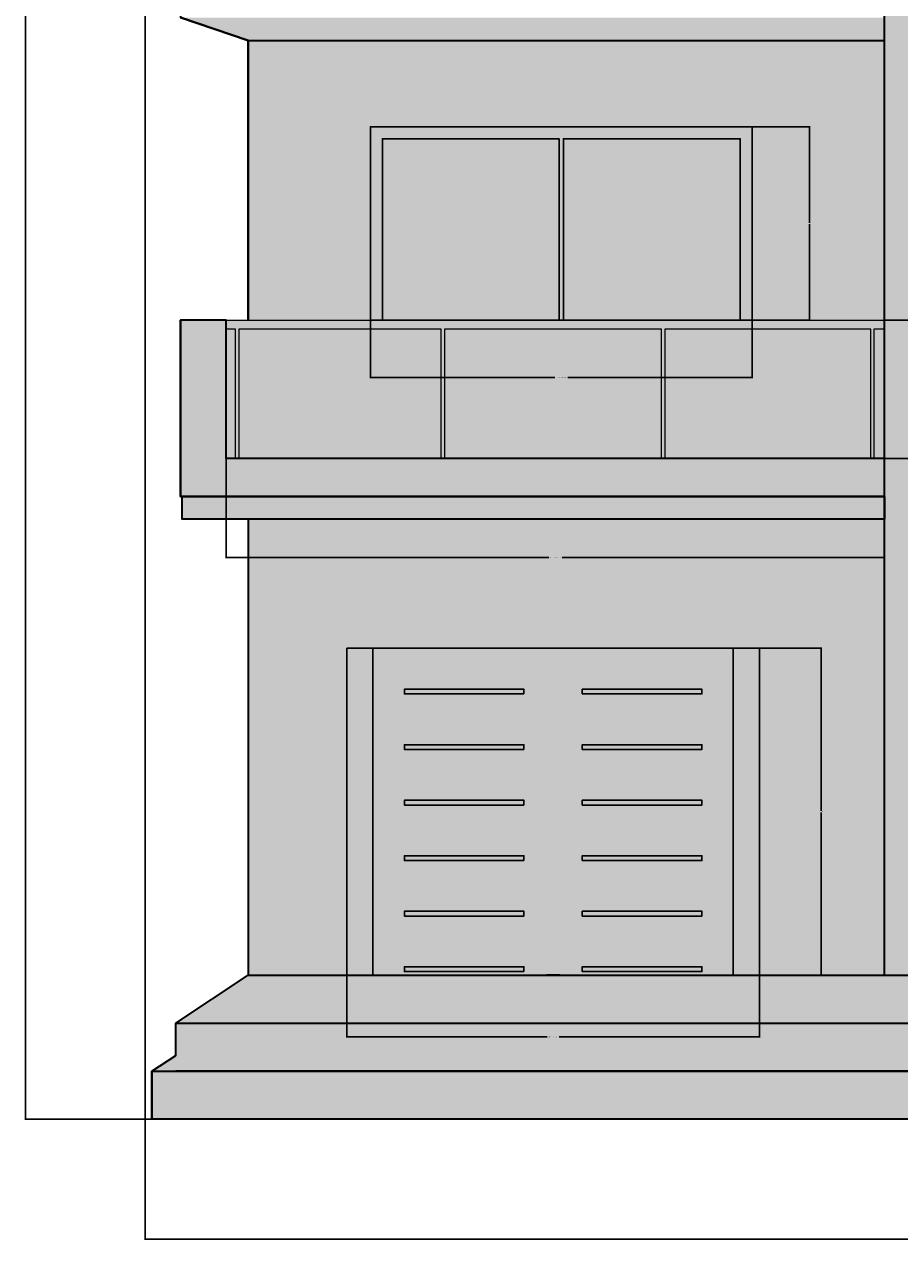
# Model space of a CAD drawing. Units: feet. Extents: x 2893 to 4112, y 897 to 1573.
# Tile 1 of 7: x 2893 to 3123, y 897 to 1217. Entities that reach past the tile are written whole.
import ezdxf

# ---------------------------------------------------------------- set-up
doc = ezdxf.new("R2010")
doc.units = ezdxf.units.FT
for name, color, linetype, lineweight in [('A-ANNO-DIMS', 2, 'Continuous', 18), ('A-DOOR', 3, 'Continuous', 25), ('A-ELEV', 7, 'Continuous', 35), ('A-ELEV-PATT', 8, 'Continuous', 13), ('A-ELEV-RAIL', 4, 'Continuous', 18), ('A-GLAZ', 4, 'Continuous', 25)]:
    doc.layers.add(name, color=color, linetype=linetype, lineweight=lineweight)
doc.styles.get("Standard").update_dxf_attribs({"font": 'arial.ttf'})
doc.dimstyles.get("Standard").update_dxf_attribs({"dimtxt": 0.18, "dimasz": 0.18, "dimexe": 0.18, "dimexo": 0.0625, "dimgap": 0.09, "dimtad": 0, "dimtih": 1, "dimtoh": 1, "dimdec": 1, "dimzin": 0, "dimdsep": 46, "dimlunit": 3, "dimtxsty": 'Standard', "dimcen": 0.09, "dimadec": 0, "dimazin": 0, "dimtfac": 1, "dimtdec": 1, "dimtofl": 0, "dimtmove": 0, "dimatfit": 3, "dimfxl": 1, "dimtolj": 1, "dimtzin": 0, "dimarcsym": 0})

# ---------------------------------------------------------------- blocks, each defined once
blk = doc.blocks.new('WIN-SLIDING')
blk.add_lwpolyline([(100.48, 0), (0, 0), (0, 50.91), (100.48, 50.91)], close=True)
blk.add_lwpolyline([(100.48, 0), (0, 0), (0, 50.91), (100.48, 50.91)], close=True)
blk.add_lwpolyline([(97.33, 0), (97.33, 47.76), (50.81, 47.76), (50.81, 0), (49.67, 0), (49.67, 47.76), (3.15, 47.76), (3.15, 0)])
blk.add_lwpolyline([(97.33, 0), (97.33, 47.76), (50.81, 47.76), (50.81, 0), (49.67, 0), (49.67, 47.76), (3.15, 47.76), (3.15, 0)])
blk = doc.blocks.new('GATE-GARAGE')
for points in [[(108.58, 0), (0, 0), (0, 86.02), (108.58, 86.02)], [(108.58, 0), (0, 0), (0, 86.02), (108.58, 86.02)], [(0, 86.02), (6.87, 86.02), (6.87, 0), (0, 0)], [(0, 86.02), (6.87, 86.02), (6.87, 0), (0, 0)], [(108.58, 86.02), (101.71, 86.02), (101.71, 0), (108.58, 0)], [(108.58, 86.02), (101.71, 86.02), (101.71, 0), (108.58, 0)], [(46.6, 73.98), (15.13, 73.98), (15.13, 75.22), (46.6, 75.22)], [(46.6, 73.98), (15.13, 73.98), (15.13, 75.22), (46.6, 75.22)], [(61.97, 73.98), (93.45, 73.98), (93.45, 75.22), (61.97, 75.22)], [(61.97, 73.98), (93.45, 73.98), (93.45, 75.22), (61.97, 75.22)], [(46.6, 59.37), (15.13, 59.37), (15.13, 60.61), (46.6, 60.61)], [(46.6, 59.37), (15.13, 59.37), (15.13, 60.61), (46.6, 60.61)], [(61.97, 59.37), (93.45, 59.37), (93.45, 60.61), (61.97, 60.61)], [(61.97, 59.37), (93.45, 59.37), (93.45, 60.61), (61.97, 60.61)], [(46.6, 44.76), (15.13, 44.76), (15.13, 46), (46.6, 46)], [(46.6, 44.76), (15.13, 44.76), (15.13, 46), (46.6, 46)], [(61.97, 44.76), (93.45, 44.76), (93.45, 46), (61.97, 46)], [(61.97, 44.76), (93.45, 44.76), (93.45, 46), (61.97, 46)], [(46.6, 30.15), (15.13, 30.15), (15.13, 31.39), (46.6, 31.39)], [(46.6, 30.15), (15.13, 30.15), (15.13, 31.39), (46.6, 31.39)], [(61.97, 30.15), (93.45, 30.15), (93.45, 31.39), (61.97, 31.39)], [(61.97, 30.15), (93.45, 30.15), (93.45, 31.39), (61.97, 31.39)], [(46.6, 15.54), (15.13, 15.54), (15.13, 16.78), (46.6, 16.78)], [(46.6, 15.54), (15.13, 15.54), (15.13, 16.78), (46.6, 16.78)], [(61.97, 15.54), (93.45, 15.54), (93.45, 16.78), (61.97, 16.78)], [(61.97, 15.54), (93.45, 15.54), (93.45, 16.78), (61.97, 16.78)], [(46.6, 0.93), (15.13, 0.93), (15.13, 2.17), (46.6, 2.17)], [(46.6, 0.93), (15.13, 0.93), (15.13, 2.17), (46.6, 2.17)], [(61.97, 0.93), (93.45, 0.93), (93.45, 2.17), (61.97, 2.17)], [(61.97, 0.93), (93.45, 0.93), (93.45, 2.17), (61.97, 2.17)]]:
    blk.add_lwpolyline(points, close=True)
blk = doc.blocks.new('BALCONY-RAIL')
blk.add_lwpolyline([(56.56, 34.07), (3.3, 34.07), (3.3, 0), (2.43, 0), (2.43, 34.07), (0, 34.07), (0, 36.45), (173.25, 36.45), (173.25, 34.07), (170.48, 34.07), (170.48, 0), (169.61, 0), (169.61, 34.07), (115.47, 34.07), (115.47, 0), (114.59, 0), (114.59, 34.07), (57.43, 34.07), (57.43, 0), (56.56, 0)], close=True)
blk.add_lwpolyline([(56.56, 34.07), (3.3, 34.07), (3.3, 0), (2.43, 0), (2.43, 34.07), (0, 34.07), (0, 36.45), (173.25, 36.45), (173.25, 34.07), (170.48, 34.07), (170.48, 0), (169.61, 0), (169.61, 34.07), (115.47, 34.07), (115.47, 0), (114.59, 0), (114.59, 34.07), (57.43, 34.07), (57.43, 0), (56.56, 0)], close=True)
blk = doc.blocks.new('*D5')
at = {"layer": 'A-ANNO-DIMS', "color": 0, "lineweight": -2, "transparency": 16777216}
for p, q in [((2984.02, 1139.32), (2984.02, 1124.13)), ((3084.5, 1139.32), (3084.5, 1124.13)), ((2984.2, 1124.31), (3032.54, 1124.31)), ((3084.32, 1124.31), (3035.98, 1124.31))]:
    blk.add_line(p, q, dxfattribs=at)
at = {"layer": 'A-ANNO-DIMS', "color": 0, "transparency": 16777216}
for points in [[(2984.2, 1124.34), (2984.2, 1124.28), (2984.02, 1124.31)], [(3084.32, 1124.34), (3084.32, 1124.28), (3084.5, 1124.31)]]:
    blk.add_solid(points, dxfattribs=at)
at = {"layer": 'Defpoints', "color": 0, "transparency": 16777216}
for p in [(2984.02, 1139.38), (3084.5, 1139.38), (3084.5, 1124.31)]:
    blk.add_point(p, dxfattribs=at)
at = {"layer": 'A-ANNO-DIMS', "color": 0, "transparency": 16777216, "insert": (3034.26, 1124.31), "char_height": 0.18, "attachment_point": 5}
blk.add_mtext('\\A1;SLIDING WINDOW 100 TYP.', dxfattribs=at)
blk = doc.blocks.new('*D6')
at = {"layer": 'A-ANNO-DIMS', "color": 0, "lineweight": -2, "transparency": 16777216}
for p, q in [((3084.56, 1190.29), (3099.75, 1190.29)), ((3099.57, 1190.11), (3099.57, 1165.02)), ((3099.57, 1139.56), (3099.57, 1164.65)), ((3084.56, 1139.38), (3099.75, 1139.38))]:
    blk.add_line(p, q, dxfattribs=at)
at = {"layer": 'A-ANNO-DIMS', "color": 0, "transparency": 16777216}
for points in [[(3099.54, 1190.11), (3099.6, 1190.11), (3099.57, 1190.29)], [(3099.54, 1139.56), (3099.6, 1139.56), (3099.57, 1139.38)]]:
    blk.add_solid(points, dxfattribs=at)
at = {"layer": 'Defpoints', "color": 0, "transparency": 16777216}
for p in [(3084.5, 1190.29), (3099.57, 1190.29), (3084.5, 1139.38)]:
    blk.add_point(p, dxfattribs=at)
at = {"layer": 'A-ANNO-DIMS', "color": 0, "transparency": 16777216, "insert": (3099.57, 1164.84), "char_height": 0.18, "attachment_point": 5}
blk.add_mtext('\\A1;51 TYP.', dxfattribs=at)
blk = doc.blocks.new('*D7')
at = {"layer": 'A-ANNO-DIMS', "color": 0, "lineweight": -2, "transparency": 16777216}
for p, q in [((2946.08, 1102.87), (2946.08, 1076.76)), ((3119.33, 1102.87), (3119.33, 1076.76)), ((2946.26, 1076.94), (3030.93, 1076.94)), ((3119.15, 1076.94), (3034.47, 1076.94))]:
    blk.add_line(p, q, dxfattribs=at)
at = {"layer": 'A-ANNO-DIMS', "color": 0, "transparency": 16777216}
for points in [[(2946.26, 1076.97), (2946.26, 1076.91), (2946.08, 1076.94)], [(3119.15, 1076.97), (3119.15, 1076.91), (3119.33, 1076.94)]]:
    blk.add_solid(points, dxfattribs=at)
at = {"layer": 'Defpoints', "color": 0, "transparency": 16777216}
for p in [(2946.08, 1102.93), (3119.33, 1102.93), (3119.33, 1076.94)]:
    blk.add_point(p, dxfattribs=at)
at = {"layer": 'A-ANNO-DIMS', "color": 0, "transparency": 16777216, "insert": (3032.7, 1076.94), "char_height": 0.18, "attachment_point": 5}
blk.add_mtext('\\A1;BALCONY RAILING 173 TYP.', dxfattribs=at)
blk = doc.blocks.new('*D8')
at = {"layer": 'A-ANNO-DIMS', "color": 0, "lineweight": -2, "transparency": 16777216}
for p, q in [((3119.39, 1139.38), (3145.49, 1139.38)), ((3145.31, 1139.2), (3145.31, 1121.34)), ((3145.31, 1103.11), (3145.31, 1120.97)), ((3119.39, 1102.93), (3145.49, 1102.93))]:
    blk.add_line(p, q, dxfattribs=at)
at = {"layer": 'A-ANNO-DIMS', "color": 0, "transparency": 16777216}
for points in [[(3145.28, 1139.2), (3145.34, 1139.2), (3145.31, 1139.38)], [(3145.28, 1103.11), (3145.34, 1103.11), (3145.31, 1102.93)]]:
    blk.add_solid(points, dxfattribs=at)
at = {"layer": 'Defpoints', "color": 0, "transparency": 16777216}
for p in [(3119.33, 1139.38), (3145.31, 1139.38), (3119.33, 1102.93)]:
    blk.add_point(p, dxfattribs=at)
at = {"layer": 'A-ANNO-DIMS', "color": 0, "transparency": 16777216, "insert": (3145.31, 1121.16), "char_height": 0.18, "attachment_point": 5}
blk.add_mtext('\\A1;36 TYP.', dxfattribs=at)
blk = doc.blocks.new('*D11')
at = {"layer": 'A-ANNO-DIMS', "color": 0, "lineweight": -2, "transparency": 16777216}
for p, q in [((2977.81, 966.95), (2977.81, 950.55)), ((3086.39, 966.95), (3086.39, 950.55)), ((2977.99, 950.73), (3030.55, 950.73)), ((3086.21, 950.73), (3033.65, 950.73))]:
    blk.add_line(p, q, dxfattribs=at)
at = {"layer": 'A-ANNO-DIMS', "color": 0, "transparency": 16777216}
for points in [[(2977.99, 950.76), (2977.99, 950.7), (2977.81, 950.73)], [(3086.21, 950.76), (3086.21, 950.7), (3086.39, 950.73)]]:
    blk.add_solid(points, dxfattribs=at)
at = {"layer": 'Defpoints', "color": 0, "transparency": 16777216}
for p in [(2977.81, 967.01), (3086.39, 967.01), (3086.39, 950.73)]:
    blk.add_point(p, dxfattribs=at)
at = {"layer": 'A-ANNO-DIMS', "color": 0, "transparency": 16777216, "insert": (3032.1, 950.73), "char_height": 0.18, "attachment_point": 5}
blk.add_mtext('\\A1;GARAGE GATE 109 TYP.', dxfattribs=at)
blk = doc.blocks.new('*D12')
at = {"layer": 'A-ANNO-DIMS', "color": 0, "lineweight": -2, "transparency": 16777216}
for p, q in [((3086.45, 1053.04), (3102.86, 1053.04)), ((3102.68, 1052.86), (3102.68, 1010.21)), ((3102.68, 967.19), (3102.68, 1009.84)), ((3086.45, 967.01), (3102.86, 967.01))]:
    blk.add_line(p, q, dxfattribs=at)
at = {"layer": 'A-ANNO-DIMS', "color": 0, "transparency": 16777216}
for points in [[(3102.65, 1052.86), (3102.71, 1052.86), (3102.68, 1053.04)], [(3102.65, 967.19), (3102.71, 967.19), (3102.68, 967.01)]]:
    blk.add_solid(points, dxfattribs=at)
at = {"layer": 'Defpoints', "color": 0, "transparency": 16777216}
for p in [(3086.39, 1053.04), (3102.68, 1053.04), (3086.39, 967.01)]:
    blk.add_point(p, dxfattribs=at)
at = {"layer": 'A-ANNO-DIMS', "color": 0, "transparency": 16777216, "insert": (3102.68, 1010.03), "char_height": 0.18, "attachment_point": 5}
blk.add_mtext('\\A1;86 TYP.', dxfattribs=at)
blk = doc.blocks.new('*D48')
at = {"layer": 'A-ANNO-DIMS', "color": 0, "lineweight": -2, "transparency": 16777216}
for p, q in [((2924.72, 1491.83), (2924.72, 897.37)), ((3417.56, 1491.83), (3417.56, 897.37)), ((2924.9, 897.55), (3170.74, 897.55)), ((3417.38, 897.55), (3171.54, 897.55))]:
    blk.add_line(p, q, dxfattribs=at)
at = {"layer": 'A-ANNO-DIMS', "color": 0, "transparency": 16777216}
for points in [[(2924.9, 897.58), (2924.9, 897.52), (2924.72, 897.55)], [(3417.38, 897.58), (3417.38, 897.52), (3417.56, 897.55)]]:
    blk.add_solid(points, dxfattribs=at)
at = {"layer": 'Defpoints', "color": 0, "transparency": 16777216}
for p in [(2924.72, 1491.89), (3417.56, 1491.89), (3417.56, 897.55)]:
    blk.add_point(p, dxfattribs=at)
at = {"layer": 'A-ANNO-DIMS', "color": 0, "transparency": 16777216, "insert": (3171.14, 897.55), "char_height": 0.18, "attachment_point": 5}
blk.add_mtext('\\A1;492.8', dxfattribs=at)
blk = doc.blocks.new('*D55')
at = {"layer": 'A-ANNO-DIMS', "color": 0, "lineweight": -2, "transparency": 16777216}
for p, q in [((2924.66, 1527.89), (2893.04, 1527.89)), ((2893.22, 1527.71), (2893.22, 1228.65)), ((2893.22, 929.23), (2893.22, 1228.29)), ((2926.44, 929.05), (2893.04, 929.05))]:
    blk.add_line(p, q, dxfattribs=at)
at = {"layer": 'A-ANNO-DIMS', "color": 0, "transparency": 16777216}
for points in [[(2893.19, 1527.71), (2893.25, 1527.71), (2893.22, 1527.89)], [(2893.19, 929.23), (2893.25, 929.23), (2893.22, 929.05)]]:
    blk.add_solid(points, dxfattribs=at)
at = {"layer": 'Defpoints', "color": 0, "transparency": 16777216}
for p in [(2893.22, 1527.89), (2924.72, 1527.89), (2926.51, 929.05)]:
    blk.add_point(p, dxfattribs=at)
at = {"layer": 'A-ANNO-DIMS', "color": 0, "transparency": 16777216, "insert": (2893.22, 1228.47), "char_height": 0.18, "attachment_point": 5}
blk.add_mtext('\\A1;598.8', dxfattribs=at)

msp = doc.modelspace()

# ---------------------------------------------------------------- hatches: boundary and pattern name
at = {"layer": 'A-ELEV-PATT'}
h = msp.add_hatch(color=256, dxfattribs=at)
h.dxf.hatch_style = 1
h.paths.add_polyline_path([(3222.9589, 1541.1646), (3119.3255, 1541.1646), (3119.3255, 967.0143), (3127.3151, 967.0143), (3127.3151, 1087.0143), (3214.9693, 1087.0143), (3214.9693, 1078.6766), (3214.9693, 967.0143), (3222.9589, 967.0143)])
h.paths.add_polyline_path([(3152.9675, 1482.3616), (3189.3169, 1482.3616), (3189.3169, 1457.0324), (3189.3169, 1377.2236), (3152.9675, 1377.2236), (3152.9675, 1457.0324)], flags=16)
h.paths.add_polyline_path([(3155.237, 1480.0922), (3187.0474, 1480.0922), (3187.0474, 1459.3019), (3155.237, 1459.3019)], flags=0)
h.paths.add_polyline_path([(3155.237, 1454.7629), (3187.0474, 1454.7629), (3187.0474, 1379.4931), (3155.237, 1379.4931)], flags=0)
h.paths.add_polyline_path([(3152.9675, 1354.8437), (3189.3169, 1354.8437), (3189.3169, 1329.5145), (3189.3169, 1249.7057), (3152.9675, 1249.7057), (3152.9675, 1329.5145)], flags=16)
h.paths.add_polyline_path([(3155.237, 1352.5742), (3187.0474, 1352.5742), (3187.0474, 1331.784), (3155.237, 1331.784)], flags=0)
h.paths.add_polyline_path([(3155.237, 1327.245), (3187.0474, 1327.245), (3187.0474, 1251.9752), (3155.237, 1251.9752)], flags=0)
h.paths.add_polyline_path([(3152.9675, 1217.2478), (3189.3169, 1217.2478), (3189.3169, 1191.9186), (3189.3169, 1112.1098), (3152.9675, 1112.1098), (3152.9675, 1191.9186)], flags=16)
h.paths.add_polyline_path([(3155.237, 1214.9783), (3187.0474, 1214.9783), (3187.0474, 1194.1881), (3155.237, 1194.1881)], flags=0)
h.paths.add_polyline_path([(3155.237, 1189.6491), (3187.0474, 1189.6491), (3187.0474, 1114.3793), (3155.237, 1114.3793)], flags=0)
h = msp.add_hatch(dxfattribs=at)
h.set_pattern_fill('AR-BRELM', color=256, scale=0.1)
h.set_pattern_definition([(0, (-663.002, 0), (0, 13.5484), [19.3675, -0.9525]), (0, (-663.002, 5.715), (0, 13.5484), [19.3675, -0.9525]), (0, (-657.922, 6.774), (0, 13.5484), [9.2075, -0.9525]), (0, (-657.922, 12.489), (0, 13.5484), [9.2075, -0.9525]), (90, (-663.002, 0), (-20.32, 1e-15), [5.715, -7.8334]), (90, (-663.954, 0), (-20.32, 1e-15), [5.715, -7.8334]), (90, (-657.922, 6.774), (-10.16, 6e-16), [5.715, -7.8334]), (90, (-658.874, 6.774), (-10.16, 6e-16), [5.715, -7.8334])])
h.paths.add_polyline_path([(3222.9589, 1541.1646), (3119.3255, 1541.1646), (3119.3255, 967.0143), (3127.3151, 967.0143), (3127.3151, 1087.0143), (3214.9693, 1087.0143), (3214.9693, 1078.6766), (3214.9693, 967.0143), (3222.9589, 967.0143)])
h.paths.add_polyline_path([(3152.9675, 1482.3616), (3189.3169, 1482.3616), (3189.3169, 1457.0324), (3189.3169, 1377.2236), (3152.9675, 1377.2236), (3152.9675, 1457.0324)], flags=16)
h.paths.add_polyline_path([(3155.237, 1480.0922), (3187.0474, 1480.0922), (3187.0474, 1459.3019), (3155.237, 1459.3019)], flags=0)
h.paths.add_polyline_path([(3155.237, 1454.7629), (3187.0474, 1454.7629), (3187.0474, 1379.4931), (3155.237, 1379.4931)], flags=0)
h.paths.add_polyline_path([(3152.9675, 1354.8437), (3189.3169, 1354.8437), (3189.3169, 1329.5145), (3189.3169, 1249.7057), (3152.9675, 1249.7057), (3152.9675, 1329.5145)], flags=16)
h.paths.add_polyline_path([(3155.237, 1352.5742), (3187.0474, 1352.5742), (3187.0474, 1331.784), (3155.237, 1331.784)], flags=0)
h.paths.add_polyline_path([(3155.237, 1327.245), (3187.0474, 1327.245), (3187.0474, 1251.9752), (3155.237, 1251.9752)], flags=0)
h.paths.add_polyline_path([(3152.9675, 1217.2478), (3189.3169, 1217.2478), (3189.3169, 1191.9186), (3189.3169, 1112.1098), (3152.9675, 1112.1098), (3152.9675, 1191.9186)], flags=16)
h.paths.add_polyline_path([(3155.237, 1214.9783), (3187.0474, 1214.9783), (3187.0474, 1194.1881), (3155.237, 1194.1881)], flags=0)
h.paths.add_polyline_path([(3155.237, 1189.6491), (3187.0474, 1189.6491), (3187.0474, 1114.3793), (3155.237, 1114.3793)], flags=0)
h = msp.add_hatch(color=256, dxfattribs=at)
h.dxf.hatch_style = 1
h.paths.add_polyline_path([(3119.3255, 1527.889), (2924.7207, 1527.889), (2924.7207, 1491.889), (3119.3255, 1491.889)])
h.paths.add_polyline_path([(3417.5637, 1527.889), (3222.9589, 1527.889), (3222.9589, 1491.889), (3417.5637, 1491.889)])
h.paths.add_polyline_path([(3119.3255, 1102.9302), (2946.0771, 1102.9302), (2946.0771, 1139.3799), (2934.0287, 1139.3799), (2934.0287, 1093.0143), (3119.3255, 1093.0143)])
h.paths.add_polyline_path([(3119.3255, 1093.0143), (2934.4679, 1093.0143), (2934.4679, 1087.0143), (3119.3255, 1087.0143)])
h.paths.add_polyline_path([(3408.2557, 1139.3799), (3396.2073, 1139.3799), (3396.2073, 1136.9984), (3396.2073, 1102.9302), (3222.9589, 1102.9302), (3222.9589, 1093.0143), (3408.2557, 1093.0143)])
h.paths.add_polyline_path([(3407.8165, 1093.0143), (3222.9589, 1093.0143), (3222.9589, 1087.0143), (3407.8165, 1087.0143)])
h = msp.add_hatch(color=256, dxfattribs=at)
h.dxf.hatch_style = 1
h.paths.add_polyline_path([(3119.3255, 1491.889), (2924.7207, 1491.889), (2945.7801, 1471.0143), (3119.3255, 1471.0143)])
h.paths.add_polyline_path([(3119.3255, 1471.0143), (2945.7801, 1471.0143), (2951.8333, 1465.0143), (3119.3255, 1465.0143)])
h.paths.add_polyline_path([(3119.3255, 1465.0143), (2951.8333, 1465.0143), (2951.8333, 1381.4641), (2984.02, 1381.4641), (2984.02, 1432.3761), (3084.4999, 1432.3761), (3084.4999, 1381.4641), (3119.3255, 1381.4641)])
h.paths.add_polyline_path([(3417.5637, 1491.889), (3222.9589, 1491.889), (3222.9589, 1471.0143), (3396.5042, 1471.0143)])
h.paths.add_polyline_path([(3396.5042, 1471.0143), (3222.9589, 1471.0143), (3222.9589, 1465.0143), (3390.4511, 1465.0143)])
h.paths.add_polyline_path([(3390.4511, 1465.0143), (3222.9589, 1465.0143), (3222.9589, 1381.4641), (3257.7845, 1381.4641), (3257.7845, 1432.3761), (3358.2644, 1432.3761), (3358.2644, 1381.4641), (3390.4511, 1381.4641)])
h.paths.add_polyline_path([(3119.3255, 1339.0143), (2942.6825, 1339.0143), (2942.6825, 1232.1197), (2948.5078, 1232.1197), (2948.5078, 1266.188), (2946.0771, 1266.188), (2946.0771, 1268.5695), (2984.02, 1268.5695), (2984.02, 1319.4815), (3084.4999, 1319.4815), (3084.4999, 1268.5695), (3119.3255, 1268.5695)], flags=17)
h.paths.add_polyline_path([(3399.6019, 1339.0143), (3222.9589, 1339.0143), (3222.9589, 1268.5695), (3257.7845, 1268.5695), (3257.7845, 1319.4815), (3358.2644, 1319.4815), (3358.2644, 1268.5695), (3396.2073, 1268.5695), (3396.2073, 1266.188), (3393.7766, 1266.188), (3393.7766, 1232.1197), (3399.6019, 1232.1197)], flags=17)
h.paths.add_polyline_path([(2942.6825, 1339.0143), (3119.3255, 1339.0143), (3119.3255, 1345.0143), (2933.3946, 1345.0143), (2933.3946, 1232.1197), (2933.3946, 1220.0947), (3119.3255, 1220.0947), (3119.3255, 1232.1197), (2942.6825, 1232.1197)])
h.paths.add_polyline_path([(3408.8898, 1345.0143), (3222.9589, 1345.0143), (3222.9589, 1339.0143), (3399.6019, 1339.0143), (3399.6019, 1232.1197), (3393.7766, 1232.1197), (3392.9028, 1232.1197), (3222.9589, 1232.1197), (3222.9589, 1220.0947), (3408.8898, 1220.0947), (3408.8898, 1232.1197)])
h.paths.add_polyline_path([(2984.02, 1190.2919), (3084.4999, 1190.2919), (3084.4999, 1139.3799), (3119.3255, 1139.3799), (3119.3255, 1213.0143), (2951.8333, 1213.0143), (2951.8333, 1139.3799), (2984.02, 1139.3799)])
h.paths.add_polyline_path([(3119.3255, 1219.0143), (2934.0287, 1219.0143), (2951.8333, 1213.0143), (3119.3255, 1213.0143)])
h.paths.add_polyline_path([(3390.4511, 1213.0143), (3222.9589, 1213.0143), (3222.9589, 1139.3799), (3257.7845, 1139.3799), (3257.7845, 1190.2919), (3358.2644, 1190.2919), (3358.2644, 1139.3799), (3390.4511, 1139.3799)])
h.paths.add_polyline_path([(3408.2557, 1219.0143), (3222.9589, 1219.0143), (3222.9589, 1213.0143), (3408.2557, 1213.0143)])
h = msp.add_hatch(color=256, dxfattribs=at)
h.dxf.hatch_style = 1
h.paths.add_polyline_path([(3119.3255, 1139.3799), (2946.0771, 1139.3799), (2946.0771, 1136.9984), (2948.5078, 1136.9984), (2948.5078, 1102.9302), (2949.3816, 1102.9302), (2949.3816, 1136.9984), (3002.6337, 1136.9984), (3002.6337, 1102.9302), (3003.5075, 1102.9302), (3003.5075, 1136.9984), (3060.6708, 1136.9984), (3060.6708, 1102.9302), (3061.5445, 1102.9302), (3061.5445, 1136.9984), (3115.685, 1136.9984), (3115.685, 1102.9302), (3116.5588, 1102.9302), (3116.5588, 1136.9984), (3119.3255, 1136.9984)])
h.paths.add_polyline_path([(2987.1701, 1187.1419), (3033.6877, 1187.1419), (3033.6877, 1139.3799), (3034.8322, 1139.3799), (3034.8322, 1187.1419), (3081.3499, 1187.1419), (3081.3499, 1139.3799), (3084.4999, 1139.3799), (3084.4999, 1190.2919), (2984.02, 1190.2919), (2984.02, 1139.3799), (2987.1701, 1139.3799)])
h.paths.add_polyline_path([(2987.1701, 1316.3314), (3033.6877, 1316.3314), (3033.6877, 1268.5695), (3034.8322, 1268.5695), (3034.8322, 1316.3314), (3081.3499, 1316.3314), (3081.3499, 1268.5695), (3084.4999, 1268.5695), (3084.4999, 1319.4815), (2984.02, 1319.4815), (2984.02, 1268.5695), (2987.1701, 1268.5695)])
h.paths.add_polyline_path([(3003.5075, 1266.188), (3060.6708, 1266.188), (3060.6708, 1232.1197), (3061.5445, 1232.1197), (3061.5445, 1266.188), (3115.685, 1266.188), (3115.685, 1232.1197), (3116.5588, 1232.1197), (3116.5588, 1266.188), (3119.3255, 1266.188), (3119.3255, 1268.5695), (2946.0771, 1268.5695), (2946.0771, 1266.188), (2948.5078, 1266.188), (2948.5078, 1232.1197), (2949.3816, 1232.1197), (2949.3816, 1266.188), (3002.6337, 1266.188), (3002.6337, 1232.1197), (3003.5075, 1232.1197)])
h.paths.add_polyline_path([(2987.1701, 1429.226), (3033.6877, 1429.226), (3033.6877, 1381.4641), (3034.8322, 1381.4641), (3034.8322, 1429.226), (3081.3499, 1429.226), (3081.3499, 1381.4641), (3084.4999, 1381.4641), (3084.4999, 1432.3761), (2984.02, 1432.3761), (2984.02, 1381.4641), (2987.1701, 1381.4641)])
h.paths.add_polyline_path([(3119.3255, 1381.4641), (2946.0771, 1381.4641), (2946.0771, 1379.0826), (2948.5078, 1379.0826), (2948.5078, 1345.0143), (2949.3816, 1345.0143), (2949.3816, 1379.0826), (3002.6337, 1379.0826), (3002.6337, 1345.0143), (3003.5075, 1345.0143), (3003.5075, 1379.0826), (3060.6708, 1379.0826), (3060.6708, 1345.0143), (3061.5445, 1345.0143), (3061.5445, 1379.0826), (3115.685, 1379.0826), (3115.685, 1345.0143), (3116.5588, 1345.0143), (3116.5588, 1379.0826), (3119.3255, 1379.0826)])
h.paths.add_polyline_path([(3189.3169, 1482.3616), (3152.9675, 1482.3616), (3152.9675, 1457.0324), (3189.3169, 1457.0324)])
h.paths.add_polyline_path([(3155.237, 1480.0922), (3187.0474, 1480.0922), (3187.0474, 1459.3019), (3155.237, 1459.3019)], flags=16)
h.paths.add_polyline_path([(3189.3169, 1457.0324), (3152.9675, 1457.0324), (3152.9675, 1377.2236), (3189.3169, 1377.2236)])
h.paths.add_polyline_path([(3155.237, 1454.7629), (3187.0474, 1454.7629), (3187.0474, 1379.4931), (3155.237, 1379.4931)], flags=16)
h.paths.add_polyline_path([(3358.2644, 1432.3761), (3257.7845, 1432.3761), (3257.7845, 1381.4641), (3260.9345, 1381.4641), (3260.9345, 1429.226), (3307.4522, 1429.226), (3307.4522, 1381.4641), (3308.5967, 1381.4641), (3308.5967, 1429.226), (3355.1143, 1429.226), (3355.1143, 1381.4641), (3358.2644, 1381.4641)])
h.paths.add_polyline_path([(3396.2073, 1381.4641), (3222.9589, 1381.4641), (3222.9589, 1379.0826), (3225.7256, 1379.0826), (3225.7256, 1345.0143), (3226.5994, 1345.0143), (3226.5994, 1379.0826), (3280.7398, 1379.0826), (3280.7398, 1345.0143), (3281.6136, 1345.0143), (3281.6136, 1379.0826), (3338.7769, 1379.0826), (3338.7769, 1345.0143), (3339.6507, 1345.0143), (3339.6507, 1379.0826), (3392.9028, 1379.0826), (3392.9028, 1345.0143), (3393.7766, 1345.0143), (3393.7766, 1379.0826), (3396.2073, 1379.0826)])
h.paths.add_polyline_path([(3358.2644, 1319.4815), (3257.7845, 1319.4815), (3257.7845, 1268.5695), (3260.9345, 1268.5695), (3260.9345, 1316.3314), (3307.4522, 1316.3314), (3307.4522, 1268.5695), (3308.5967, 1268.5695), (3308.5967, 1316.3314), (3355.1143, 1316.3314), (3355.1143, 1268.5695), (3358.2644, 1268.5695)])
h.paths.add_polyline_path([(3396.2073, 1268.5695), (3222.9589, 1268.5695), (3222.9589, 1266.188), (3225.7256, 1266.188), (3225.7256, 1232.1197), (3226.5994, 1232.1197), (3226.5994, 1266.188), (3280.7398, 1266.188), (3280.7398, 1232.1197), (3281.6136, 1232.1197), (3281.6136, 1266.188), (3338.7769, 1266.188), (3338.7769, 1232.1197), (3339.6507, 1232.1197), (3339.6507, 1266.188), (3392.9028, 1266.188), (3392.9028, 1232.1197), (3393.7766, 1232.1197), (3393.7766, 1266.188), (3396.2073, 1266.188)])
h.paths.add_polyline_path([(3260.9345, 1187.1419), (3307.4522, 1187.1419), (3307.4522, 1139.3799), (3308.5967, 1139.3799), (3308.5967, 1187.1419), (3355.1143, 1187.1419), (3355.1143, 1139.3799), (3358.2644, 1139.3799), (3358.2644, 1190.2919), (3257.7845, 1190.2919), (3257.7845, 1139.3799), (3260.9345, 1139.3799)])
h.paths.add_polyline_path([(3396.2073, 1139.3799), (3222.9589, 1139.3799), (3222.9589, 1136.9984), (3225.7256, 1136.9984), (3225.7256, 1102.9302), (3226.5994, 1102.9302), (3226.5994, 1136.9984), (3280.7398, 1136.9984), (3280.7398, 1102.9302), (3281.6136, 1102.9302), (3281.6136, 1136.9984), (3338.7769, 1136.9984), (3338.7769, 1102.9302), (3339.6507, 1102.9302), (3339.6507, 1136.9984), (3392.9028, 1136.9984), (3392.9028, 1102.9302), (3393.7766, 1102.9302), (3393.7766, 1136.9984), (3396.2073, 1136.9984)])
h.paths.add_polyline_path([(3189.3169, 1354.8437), (3152.9675, 1354.8437), (3152.9675, 1329.5145), (3189.3169, 1329.5145)])
h.paths.add_polyline_path([(3155.237, 1331.784), (3155.237, 1352.5742), (3187.0474, 1352.5742), (3187.0474, 1331.784)], flags=16)
h.paths.add_polyline_path([(3189.3169, 1329.5145), (3152.9675, 1329.5145), (3152.9675, 1249.7057), (3189.3169, 1249.7057)])
h.paths.add_polyline_path([(3155.237, 1327.245), (3187.0474, 1327.245), (3187.0474, 1251.9752), (3155.237, 1251.9752)], flags=16)
h.paths.add_polyline_path([(3189.3169, 1191.9186), (3152.9675, 1191.9186), (3152.9675, 1112.1098), (3189.3169, 1112.1098)])
h.paths.add_polyline_path([(3155.237, 1189.6491), (3187.0474, 1189.6491), (3187.0474, 1114.3793), (3155.237, 1114.3793)], flags=16)
h.paths.add_polyline_path([(3189.3169, 1217.2478), (3152.9675, 1217.2478), (3152.9675, 1191.9186), (3189.3169, 1191.9186)])
h.paths.add_polyline_path([(3155.237, 1194.1881), (3155.237, 1214.9783), (3187.0474, 1214.9783), (3187.0474, 1194.1881)], flags=16)
h = msp.add_hatch(color=256, dxfattribs=at)
h.dxf.hatch_style = 1
h.paths.add_polyline_path([(3033.6877, 1429.226), (2987.1701, 1429.226), (2987.1701, 1381.4641), (3033.6877, 1381.4641)])
h.paths.add_polyline_path([(3081.3499, 1429.226), (3034.8322, 1429.226), (3034.8322, 1381.4641), (3081.3499, 1381.4641)])
h.paths.add_polyline_path([(3115.685, 1379.0826), (3061.5445, 1379.0826), (3061.5445, 1345.0143), (3115.685, 1345.0143)])
h.paths.add_polyline_path([(3119.3255, 1379.0826), (3116.5588, 1379.0826), (3116.5588, 1345.0143), (3119.3255, 1345.0143)])
h.paths.add_polyline_path([(3060.6708, 1379.0826), (3003.5075, 1379.0826), (3003.5075, 1345.0143), (3060.6708, 1345.0143)])
h.paths.add_polyline_path([(3002.6337, 1379.0826), (2949.3816, 1379.0826), (2949.3816, 1345.0143), (3002.6337, 1345.0143)])
h.paths.add_polyline_path([(2948.5078, 1379.0826), (2946.0771, 1379.0826), (2946.0771, 1345.0143), (2948.5078, 1345.0143)])
h.paths.add_polyline_path([(3355.1143, 1429.226), (3308.5967, 1429.226), (3308.5967, 1381.4641), (3355.1143, 1381.4641)])
h.paths.add_polyline_path([(3307.4522, 1429.226), (3260.9345, 1429.226), (3260.9345, 1381.4641), (3307.4522, 1381.4641)])
h.paths.add_polyline_path([(3225.7256, 1379.0826), (3222.9589, 1379.0826), (3222.9589, 1345.0143), (3225.7256, 1345.0143)])
h.paths.add_polyline_path([(3280.7398, 1379.0826), (3226.5994, 1379.0826), (3226.5994, 1345.0143), (3280.7398, 1345.0143)])
h.paths.add_polyline_path([(3338.7769, 1379.0826), (3281.6136, 1379.0826), (3281.6136, 1345.0143), (3338.7769, 1345.0143)])
h.paths.add_polyline_path([(3392.9028, 1379.0826), (3339.6507, 1379.0826), (3339.6507, 1345.0143), (3392.9028, 1345.0143)])
h.paths.add_polyline_path([(3187.0474, 1480.0922), (3155.237, 1480.0922), (3155.237, 1459.3019), (3187.0474, 1459.3019)])
h.paths.add_polyline_path([(3187.0474, 1454.7629), (3155.237, 1454.7629), (3155.237, 1379.4931), (3187.0474, 1379.4931)])
h.paths.add_polyline_path([(3187.0474, 1352.5742), (3155.237, 1352.5742), (3155.237, 1331.784), (3187.0474, 1331.784)])
h.paths.add_polyline_path([(3187.0474, 1327.245), (3155.237, 1327.245), (3155.237, 1251.9752), (3187.0474, 1251.9752)])
h.paths.add_polyline_path([(3033.6877, 1316.3314), (2987.1701, 1316.3314), (2987.1701, 1268.5695), (3033.6877, 1268.5695)])
h.paths.add_polyline_path([(3081.3499, 1316.3314), (3034.8322, 1316.3314), (3034.8322, 1268.5695), (3081.3499, 1268.5695)])
h.paths.add_polyline_path([(3002.6337, 1266.188), (2949.3816, 1266.188), (2949.3816, 1232.1197), (3002.6337, 1232.1197)])
h.paths.add_polyline_path([(3060.6708, 1266.188), (3003.5075, 1266.188), (3003.5075, 1232.1197), (3060.6708, 1232.1197)])
h.paths.add_polyline_path([(3115.685, 1266.188), (3061.5445, 1266.188), (3061.5445, 1232.1197), (3115.685, 1232.1197)])
h.paths.add_polyline_path([(3119.3255, 1266.188), (3116.5588, 1266.188), (3116.5588, 1232.1197), (3119.3255, 1232.1197)])
h.paths.add_polyline_path([(3307.4522, 1316.3314), (3260.9345, 1316.3314), (3260.9345, 1268.5695), (3307.4522, 1268.5695)])
h.paths.add_polyline_path([(3355.1143, 1316.3314), (3308.5967, 1316.3314), (3308.5967, 1268.5695), (3355.1143, 1268.5695)])
h.paths.add_polyline_path([(3392.9028, 1266.188), (3339.6507, 1266.188), (3339.6507, 1232.1197), (3392.9028, 1232.1197)])
h.paths.add_polyline_path([(3338.7769, 1266.188), (3281.6136, 1266.188), (3281.6136, 1232.1197), (3338.7769, 1232.1197)])
h.paths.add_polyline_path([(3280.7398, 1266.188), (3226.5994, 1266.188), (3226.5994, 1232.1197), (3280.7398, 1232.1197)])
h.paths.add_polyline_path([(3225.7256, 1266.188), (3222.9589, 1266.188), (3222.9589, 1232.1197), (3225.7256, 1232.1197)])
h.paths.add_polyline_path([(3033.6877, 1187.1419), (2987.1701, 1187.1419), (2987.1701, 1139.3799), (3033.6877, 1139.3799)])
h.paths.add_polyline_path([(3081.3499, 1187.1419), (3034.8322, 1187.1419), (3034.8322, 1139.3799), (3081.3499, 1139.3799)])
h.paths.add_polyline_path([(3002.6337, 1136.9984), (2949.3816, 1136.9984), (2949.3816, 1102.9302), (3002.6337, 1102.9302)])
h.paths.add_polyline_path([(3060.6708, 1136.9984), (3003.5075, 1136.9984), (3003.5075, 1102.9302), (3060.6708, 1102.9302)])
h.paths.add_polyline_path([(3115.685, 1136.9984), (3061.5445, 1136.9984), (3061.5445, 1102.9302), (3115.685, 1102.9302)])
h.paths.add_polyline_path([(3187.0474, 1214.9783), (3155.237, 1214.9783), (3155.237, 1194.1881), (3187.0474, 1194.1881)])
h.paths.add_polyline_path([(3187.0474, 1189.6491), (3155.237, 1189.6491), (3155.237, 1114.3793), (3187.0474, 1114.3793)])
h.paths.add_polyline_path([(3307.4522, 1187.1419), (3260.9345, 1187.1419), (3260.9345, 1139.3799), (3307.4522, 1139.3799)])
h.paths.add_polyline_path([(3355.1143, 1187.1419), (3308.5967, 1187.1419), (3308.5967, 1139.3799), (3355.1143, 1139.3799)])
h.paths.add_polyline_path([(3280.7398, 1136.9984), (3226.5994, 1136.9984), (3226.5994, 1102.9302), (3280.7398, 1102.9302)])
h.paths.add_polyline_path([(3338.7769, 1136.9984), (3281.6136, 1136.9984), (3281.6136, 1102.9302), (3338.7769, 1102.9302)])
h.paths.add_polyline_path([(3392.9028, 1136.9984), (3339.6507, 1136.9984), (3339.6507, 1102.9302), (3392.9028, 1102.9302)])
h.paths.add_polyline_path([(3225.7256, 1136.9984), (3222.9589, 1136.9984), (3222.9589, 1102.9302), (3225.7256, 1102.9302)])
h.paths.add_polyline_path([(3119.3255, 1136.9984), (3116.5588, 1136.9984), (3116.5588, 1102.9302), (3119.3255, 1102.9302)])
h.paths.add_polyline_path([(2948.5078, 1136.9984), (2946.0771, 1136.9984), (2946.0771, 1102.9302), (2948.5078, 1102.9302)])
h.paths.add_polyline_path([(3396.2073, 1136.9984), (3393.7766, 1136.9984), (3393.7766, 1102.9302), (3396.2073, 1102.9302)])
h = msp.add_hatch(color=256, dxfattribs=at)
h.dxf.hatch_style = 1
h.paths.add_polyline_path([(3390.4511, 1087.0143), (3222.9589, 1087.0143), (3222.9589, 967.0143), (3255.8959, 967.0143), (3255.8959, 1053.0375), (3262.7641, 1053.0375), (3364.4735, 1053.0375), (3364.4735, 967.0143), (3390.4511, 967.0143)])
h.paths.add_polyline_path([(3119.3255, 1087.0143), (2951.8333, 1087.0143), (2951.8333, 967.0143), (2977.8109, 967.0143), (2977.8109, 1053.0375), (2984.6791, 1053.0375), (3086.3885, 1053.0375), (3086.3885, 967.0143), (3119.3255, 967.0143)])
h = msp.add_hatch(color=256, dxfattribs=at)
h.dxf.hatch_style = 1
h.paths.add_polyline_path([(3079.5203, 1053.0375), (2984.6791, 1053.0375), (2984.6791, 967.0143), (3079.5203, 967.0143)])
h.paths.add_polyline_path([(3024.4136, 1040.9943), (2992.942, 1040.9943), (2992.942, 1042.2356), (3024.4136, 1042.2356)], flags=16)
h.paths.add_polyline_path([(3039.7858, 1042.2356), (3071.2574, 1042.2356), (3071.2574, 1040.9943), (3039.7858, 1040.9943)], flags=16)
h.paths.add_polyline_path([(3024.4136, 1027.6246), (3024.4136, 1026.3833), (2992.942, 1026.3833), (2992.942, 1027.6246)], flags=16)
h.paths.add_polyline_path([(3039.7858, 1027.6246), (3071.2574, 1027.6246), (3071.2574, 1026.3833), (3039.7858, 1026.3833)], flags=16)
h.paths.add_polyline_path([(3024.4136, 1013.0137), (3024.4136, 1011.7724), (2992.942, 1011.7724), (2992.942, 1013.0137)], flags=16)
h.paths.add_polyline_path([(3039.7858, 1013.0137), (3071.2574, 1013.0137), (3071.2574, 1011.7724), (3039.7858, 1011.7724)], flags=16)
h.paths.add_polyline_path([(3024.4136, 998.4028), (3024.4136, 997.1615), (2992.942, 997.1615), (2992.942, 998.4028)], flags=16)
h.paths.add_polyline_path([(3039.7858, 998.4028), (3071.2574, 998.4028), (3071.2574, 997.1615), (3039.7858, 997.1615)], flags=16)
h.paths.add_polyline_path([(3024.4136, 983.7919), (3024.4136, 982.5506), (2992.942, 982.5506), (2992.942, 983.7919)], flags=16)
h.paths.add_polyline_path([(3039.7858, 983.7919), (3071.2574, 983.7919), (3071.2574, 982.5506), (3039.7858, 982.5506)], flags=16)
h.paths.add_polyline_path([(3024.4136, 969.181), (3024.4136, 967.9397), (2992.942, 967.9397), (2992.942, 969.181)], flags=16)
h.paths.add_polyline_path([(3039.7858, 969.181), (3071.2574, 969.181), (3071.2574, 967.9397), (3039.7858, 967.9397)], flags=16)
h.paths.add_polyline_path([(3086.3885, 1053.0375), (3079.5203, 1053.0375), (3079.5203, 967.0143), (3086.3885, 967.0143)])
h.paths.add_polyline_path([(3364.4735, 1053.0375), (3357.6053, 1053.0375), (3357.6053, 967.0143), (3364.4735, 967.0143)])
h.paths.add_polyline_path([(3357.6053, 1053.0375), (3262.7641, 1053.0375), (3262.7641, 967.0143), (3357.6053, 967.0143)])
h.paths.add_polyline_path([(3271.027, 1026.3833), (3271.027, 1027.6246), (3302.4986, 1027.6246), (3302.4986, 1026.3833)], flags=16)
h.paths.add_polyline_path([(3271.027, 1013.0137), (3302.4986, 1013.0137), (3302.4986, 1011.7724), (3271.027, 1011.7724)], flags=16)
h.paths.add_polyline_path([(3271.027, 1040.9943), (3271.027, 1042.2356), (3302.4986, 1042.2356), (3302.4986, 1040.9943)], flags=16)
h.paths.add_polyline_path([(3271.027, 998.4028), (3302.4986, 998.4028), (3302.4986, 997.1615), (3271.027, 997.1615)], flags=16)
h.paths.add_polyline_path([(3271.027, 983.7919), (3302.4986, 983.7919), (3302.4986, 982.5506), (3271.027, 982.5506)], flags=16)
h.paths.add_polyline_path([(3317.8708, 1026.3833), (3317.8708, 1027.6246), (3349.3424, 1027.6246), (3349.3424, 1026.3833)], flags=16)
h.paths.add_polyline_path([(3317.8708, 1013.0137), (3349.3424, 1013.0137), (3349.3424, 1011.7724), (3317.8708, 1011.7724)], flags=16)
h.paths.add_polyline_path([(3271.027, 969.181), (3302.4986, 969.181), (3302.4986, 967.9397), (3271.027, 967.9397)], flags=16)
h.paths.add_polyline_path([(3317.8708, 1040.9943), (3317.8708, 1042.2356), (3349.3424, 1042.2356), (3349.3424, 1040.9943)], flags=16)
h.paths.add_polyline_path([(3317.8708, 998.4028), (3349.3424, 998.4028), (3349.3424, 997.1615), (3317.8708, 997.1615)], flags=16)
h.paths.add_polyline_path([(3317.8708, 983.7919), (3349.3424, 983.7919), (3349.3424, 982.5506), (3317.8708, 982.5506)], flags=16)
h.paths.add_polyline_path([(3317.8708, 969.181), (3349.3424, 969.181), (3349.3424, 967.9397), (3317.8708, 967.9397)], flags=16)
h.paths.add_polyline_path([(3262.7641, 1053.0375), (3255.8959, 1053.0375), (3255.8959, 967.0143), (3262.7641, 967.0143)])
h.paths.add_polyline_path([(2984.6791, 1053.0375), (2977.8109, 1053.0375), (2977.8109, 967.0143), (2984.6791, 967.0143)])
h = msp.add_hatch(color=256, dxfattribs=at)
h.dxf.hatch_style = 1
h.paths.add_polyline_path([(3024.4136, 1042.2356), (2992.942, 1042.2356), (2992.942, 1040.9943), (3024.4136, 1040.9943)])
h.paths.add_polyline_path([(3071.2574, 1042.2356), (3039.7858, 1042.2356), (3039.7858, 1040.9943), (3071.2574, 1040.9943)])
h.paths.add_polyline_path([(3024.4136, 1027.6246), (2992.942, 1027.6246), (2992.942, 1026.3833), (3024.4136, 1026.3833)])
h.paths.add_polyline_path([(3071.2574, 1027.6246), (3039.7858, 1027.6246), (3039.7858, 1026.3833), (3071.2574, 1026.3833)])
h.paths.add_polyline_path([(3024.4136, 1013.0137), (2992.942, 1013.0137), (2992.942, 1011.7724), (3024.4136, 1011.7724)])
h.paths.add_polyline_path([(3071.2574, 1013.0137), (3039.7858, 1013.0137), (3039.7858, 1011.7724), (3071.2574, 1011.7724)])
h.paths.add_polyline_path([(3024.4136, 998.4028), (2992.942, 998.4028), (2992.942, 997.1615), (3024.4136, 997.1615)])
h.paths.add_polyline_path([(3071.2574, 998.4028), (3039.7858, 998.4028), (3039.7858, 997.1615), (3071.2574, 997.1615)])
h.paths.add_polyline_path([(3024.4136, 983.7919), (2992.942, 983.7919), (2992.942, 982.5506), (3024.4136, 982.5506)])
h.paths.add_polyline_path([(3071.2574, 983.7919), (3039.7858, 983.7919), (3039.7858, 982.5506), (3071.2574, 982.5506)])
h.paths.add_polyline_path([(3071.2574, 969.181), (3039.7858, 969.181), (3039.7858, 967.9397), (3071.2574, 967.9397)])
h.paths.add_polyline_path([(3024.4136, 969.181), (2992.942, 969.181), (2992.942, 967.9397), (3024.4136, 967.9397)])
h.paths.add_polyline_path([(3302.4986, 1042.2356), (3271.027, 1042.2356), (3271.027, 1040.9943), (3302.4986, 1040.9943)])
h.paths.add_polyline_path([(3349.3424, 1042.2356), (3317.8708, 1042.2356), (3317.8708, 1040.9943), (3349.3424, 1040.9943)])
h.paths.add_polyline_path([(3302.4986, 1027.6246), (3271.027, 1027.6246), (3271.027, 1026.3833), (3302.4986, 1026.3833)])
h.paths.add_polyline_path([(3349.3424, 1027.6246), (3317.8708, 1027.6246), (3317.8708, 1026.3833), (3349.3424, 1026.3833)])
h.paths.add_polyline_path([(3302.4986, 1013.0137), (3271.027, 1013.0137), (3271.027, 1011.7724), (3302.4986, 1011.7724)])
h.paths.add_polyline_path([(3349.3424, 1013.0137), (3317.8708, 1013.0137), (3317.8708, 1011.7724), (3349.3424, 1011.7724)])
h.paths.add_polyline_path([(3302.4986, 998.4028), (3271.027, 998.4028), (3271.027, 997.1615), (3302.4986, 997.1615)])
h.paths.add_polyline_path([(3349.3424, 998.4028), (3317.8708, 998.4028), (3317.8708, 997.1615), (3349.3424, 997.1615)])
h.paths.add_polyline_path([(3302.4986, 983.7919), (3271.027, 983.7919), (3271.027, 982.5506), (3302.4986, 982.5506)])
h.paths.add_polyline_path([(3349.3424, 983.7919), (3317.8708, 983.7919), (3317.8708, 982.5506), (3349.3424, 982.5506)])
h.paths.add_polyline_path([(3302.4986, 969.181), (3271.027, 969.181), (3271.027, 967.9397), (3302.4986, 967.9397)])
h.paths.add_polyline_path([(3349.3424, 969.181), (3317.8708, 969.181), (3317.8708, 967.9397), (3349.3424, 967.9397)])
h = msp.add_hatch(color=256, dxfattribs=at)
h.dxf.hatch_style = 1
h.paths.add_polyline_path([(3390.4511, 967.0143), (3222.9589, 967.0143), (2951.8333, 967.0143), (2932.7702, 954.3595), (3409.5142, 954.3595)])
h.paths.add_polyline_path([(3409.5142, 954.3595), (2932.7702, 954.3595), (2932.7702, 945.8624), (2926.5072, 941.7047), (3415.7772, 941.7047), (3409.5142, 945.8624)])
h.paths.add_polyline_path([(3415.7772, 941.7047), (2926.5072, 941.7047), (2926.5072, 929.0499), (3415.7772, 929.0499)])

# ---------------------------------------------------------------- linework, layer by layer
at = {"layer": 'A-ELEV'}
for p, q in [((3119.3255, 967.0143), (3119.3255, 1541.1646)), ((2951.8333, 1213.0143), (2934.0287, 1219.0143)), ((2951.8333, 1213.0143), (3119.3255, 1213.0143)), ((2951.8333, 1139.3799), (2951.8333, 1213.0143)), ((2951.8333, 1213.0143), (2951.8333, 1139.3799)), ((2934.0287, 1093.0143), (2934.0287, 1139.3799)), ((3119.3255, 1093.0143), (2934.0287, 1093.0143)), ((3119.3255, 1087.0143), (2934.4679, 1087.0143)), ((2932.7702, 954.3595), (2951.8333, 967.0143)), ((2932.7702, 954.3595), (2951.8333, 967.0143)), ((2951.8333, 967.0143), (3390.4511, 967.0143)), ((2951.8333, 967.0143), (3390.4511, 967.0143)), ((2926.5072, 941.7047), (2932.7702, 945.8624)), ((2926.5072, 941.7047), (2926.5072, 929.0499))]:
    msp.add_line(p, q, dxfattribs=at)
for points in [[(3119.3255, 967.0143), (3119.3255, 1541.1646), (3222.9589, 1541.1646), (3222.9589, 967.0143)], [(3119.3255, 1339.0143), (2942.6825, 1339.0143), (2942.6825, 1232.1197), (3119.3255, 1232.1197), (3119.3255, 1220.0947), (2933.3946, 1220.0947), (2933.3946, 1232.1197), (2933.3946, 1345.0143), (2933.3946, 1220.0947), (2934.0287, 1220.0947), (2934.0287, 1219.0143), (2951.8333, 1213.0143), (2951.8333, 1139.3799), (2951.8333, 1213.0143), (3119.3255, 1213.0143)], [(2946.0771, 1102.9302), (2946.0771, 1139.3799), (2934.0287, 1139.3799), (2934.0287, 1093.0143)], [(2951.8333, 1087.0143), (2951.8333, 967.0143), (3119.3255, 967.0143), (3119.3255, 1087.0143), (3119.3255, 1102.9302), (2946.0771, 1102.9302), (2946.0771, 1139.3799), (2934.0287, 1139.3799), (2934.0287, 1093.0143), (2934.0287, 1102.9302)], [(2934.0287, 1139.3799), (2934.0287, 1093.0143), (3119.3255, 1093.0143), (3119.3255, 1087.0143), (2934.4679, 1087.0143), (2934.4679, 1093.0143)], [(2934.0287, 1102.9302), (2934.0287, 1093.0143)], [(3119.3255, 1087.0143), (3119.3255, 1102.9302), (2946.0771, 1102.9302)], [(2934.4679, 1087.0143), (2934.4679, 1093.0143)], [(3119.3255, 1093.0143), (3119.3255, 1087.0143)], [(2951.8333, 1087.0143), (2951.8333, 967.0143), (3119.3255, 967.0143), (3119.3255, 1087.0143)], [(3033.8396, 967.0143), (3030.3598, 967.0143)], [(3033.8396, 967.0143), (3030.3598, 967.0143)], [(2932.7702, 945.8624), (2932.7702, 954.3595), (3409.5142, 954.3595), (3409.5142, 945.8624)], [(2926.5072, 941.7047), (3415.7772, 941.7047)], [(2926.5072, 941.7047), (3415.7772, 941.7047)], [(3409.5142, 941.7047), (2932.7702, 941.7047)], [(3409.5142, 941.7047), (2932.7702, 941.7047)], [(3415.7772, 929.0499), (2926.5072, 929.0499)]]:
    msp.add_lwpolyline(points, dxfattribs=at)
msp.add_lwpolyline([(2926.5072, 941.7047), (2932.7702, 945.8624), (2932.7702, 954.3595), (3409.5142, 954.3595), (3409.5142, 945.8624), (3415.7772, 941.7047), (3415.7772, 929.0499), (2926.5072, 929.0499)], close=True, dxfattribs=at)

# ---------------------------------------------------------------- block references
at = {"layer": 'A-DOOR'}
msp.add_blockref('GATE-GARAGE', (2977.811, 967.014), dxfattribs=at)
at = {"layer": 'A-ELEV-RAIL'}
msp.add_blockref('BALCONY-RAIL', (2946.077, 1102.93), dxfattribs=at)
at = {"layer": 'A-GLAZ'}
msp.add_blockref('WIN-SLIDING', (2984.02, 1139.38), dxfattribs=at)

# ---------------------------------------------------------------- dimensions: what is measured, and where the dimension line sits
at = {"layer": 'A-ANNO-DIMS'}
dim = msp.add_linear_dim(base=(2893.2207, 1527.889), p1=(2926.5072, 929.0499), p2=(2924.7207, 1527.889), angle=90, dimstyle='Standard', override={"dimdec": 1, "dimlfac": 1, "dimrnd": 0, "dimzin": 0, "dimdsep": 46, "dimlunit": 2}, dxfattribs=at)
dim.commit()
dim.dimension.update_dxf_attribs({"geometry": '*D55', "text_midpoint": (2893.2207, 1228.4695)})
dim = msp.add_linear_dim(base=(3417.5637, 897.5499), p1=(2924.7207, 1491.889), p2=(3417.5637, 1491.889), dimstyle='Standard', override={"dimdec": 1, "dimlfac": 1, "dimrnd": 0, "dimzin": 0, "dimdsep": 46, "dimlunit": 2}, dxfattribs=at)
dim.commit()
dim.dimension.update_dxf_attribs({"geometry": '*D48', "text_midpoint": (3171.1422, 897.5499)})
for base, p1, p2, picture, middle in [((3099.5719, 1190.2919), (3084.4999, 1139.3799), (3084.4999, 1190.2919), '*D6', (3099.5719, 1164.8359)), ((3145.3128, 1139.3799), (3119.3255, 1102.9302), (3119.3255, 1139.3799), '*D8', (3145.3128, 1121.1551)), ((3102.6752, 1053.0375), (3086.3885, 967.0143), (3086.3885, 1053.0375), '*D12', (3102.6752, 1010.0259))]:
    dim = msp.add_linear_dim(base=base, p1=p1, p2=p2, angle=90, text='<> TYP.', dimstyle='Standard', override={"dimdec": 0, "dimlfac": 1, "dimrnd": 0, "dimzin": 0, "dimdsep": 46, "dimlunit": 2}, dxfattribs=at)
    dim.commit()
    dim.dimension.update_dxf_attribs({"geometry": picture, "text_midpoint": middle})
for base, p1, p2, text, picture, middle in [((3084.4999, 1124.308), (2984.02, 1139.3799), (3084.4999, 1139.3799), 'SLIDING WINDOW <> TYP.', '*D5', (3034.26, 1124.308)), ((3119.3255, 1076.9429), (2946.0771, 1102.9302), (3119.3255, 1102.9302), 'BALCONY RAILING <> TYP.', '*D7', (3032.7013, 1076.9429)), ((3086.3885, 950.7277), (2977.8109, 967.0143), (3086.3885, 967.0143), 'GARAGE GATE <> TYP.', '*D11', (3032.0997, 950.7277))]:
    dim = msp.add_linear_dim(base=base, p1=p1, p2=p2, text=text, dimstyle='Standard', override={"dimdec": 0, "dimlfac": 1, "dimrnd": 0, "dimzin": 0, "dimdsep": 46, "dimlunit": 2}, dxfattribs=at)
    dim.commit()
    dim.dimension.update_dxf_attribs({"geometry": picture, "text_midpoint": middle})

doc.saveas('drawing.dxf')
